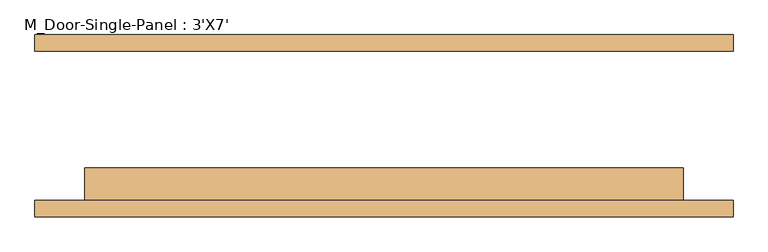
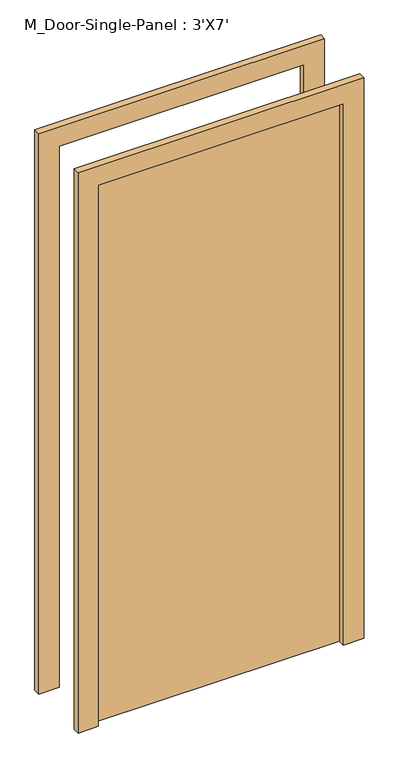
"""IFC4 building model written with IfcOpenShell, lengths in millimetres: door geometry, M_Door-Single-Panel : 3'X7'."""

from ifc_helpers import new_model, si_unit, frame, origin, origin_with_axes, place, context, project, spatial, polyline, outline, extrude, source, transform, mapped, element, save


def m_door_single_panel_3_x7_2af5d1b8(model_context):
    return source(origin(), model_context, "Body", "SweptSolid", [
        extrude(outline(polyline([(457.2, -64.3), (457.2, -114.3), (-457.2, -114.3), (-457.2, -64.3), (457.2, -64.3)])), origin_with_axes(), (0.0, 0.0, 1.0), 2133.6),
        extrude(outline(polyline([(2209.8, 533.4), (2209.8, -533.4), (0.0, -533.4), (0.0, -457.2), (2133.6, -457.2), (2133.6, 457.2), (0.0, 457.2), (0.0, 533.4), (2209.8, 533.4)])), frame((0.0, 114.3, 0.0), z_axis=(0.0, 1.0, 0.0), x_axis=(0.0, 0.0, 1.0)), (0.0, 0.0, 1.0), 25.0),
        extrude(outline(polyline([(2209.8, -533.4), (0.0, -533.4), (0.0, -457.2), (2133.6, -457.2), (2133.6, 457.2), (0.0, 457.2), (0.0, 533.4), (2209.8, 533.4), (2209.8, -533.4)])), frame((0.0, -139.3, 0.0), z_axis=(0.0, 1.0, 0.0), x_axis=(0.0, 0.0, 1.0)), (0.0, 0.0, 1.0), 25.0),
    ])


if __name__ == "__main__":
    model = new_model("IFC4")
    model_context = context("Model", 3, world=origin())
    ifc_project = project(units=[si_unit("LENGTHUNIT", "METRE", prefix="MILLI")], contexts=[model_context])
    site = spatial("IfcSite", under=ifc_project)
    building = spatial("IfcBuilding", under=site)
    placement = place(None, origin())
    m_door_single_panel_3_x7_shape = m_door_single_panel_3_x7_2af5d1b8(model_context)
    element("IfcDoor", 1, ObjectType="M_Door-Single-Panel : 3'X7'", at=placement, inside=building, context=model_context, shape_type="MappedRepresentation", body=[
        mapped(m_door_single_panel_3_x7_shape, transform((0.0, 0.0, 0.0), x_axis=(1.0, 0.0, 0.0), y_axis=(0.0, 1.0, 0.0), z_axis=(0.0, 0.0, 1.0))),
    ])
    save(model, "model.ifc")

# Revit data of these elements
# Type "M_Door-Single-Panel : 3'X7'"
#   Type Mark = "11"
#   Construction Type Id = "DOOR"
#   Assembly Code = "C1020300"
#   Analytic Construction = "Wooden"
#   Thickness = 0' - 1.9685"
#   Thermal Resistance (R) = 2.5876 (h·ft²·°F)/BTU
#   Swing Angle [instance default] = 90.00°
#   Heat Transfer Coefficient (U) = 0.3865 BTU/(h·ft²·°F)
#   Height = 7' - 0"
#   Trim Projection Ext = 0' - 0.98425"
#   Trim Projection Int = 0' - 0.98425"
#   Trim Width = 0' - 3.14961"
#   Width = 3' - 0"
#   Define Thermal Properties by = 1
#   Panel Material = Wood - Birch - Solid Stained Light Low Gloss
#   Trim Material = Paint - Sienna
#   Visual Light Transmittance = 0
#   Solar Heat Gain Coefficient = 0
#   Function = (empty or 0)
#   Wall Closure = (empty or 0)
# Element 1 (IfcDoor, "M_Door-Single-Panel : 3'X7'")
#   Materials on its faces: "Paint - Sienna", "Wood - Birch - Solid Stained Light Low Gloss"
# Materials
#   "Wood - Birch - Solid Stained Light Low Gloss": class "Wood", colour RGB 210 159 95, transparency 0, Cost = 0
#   "Paint - Sienna": colour RGB 118 70 51, transparency 0, Cost = 0
